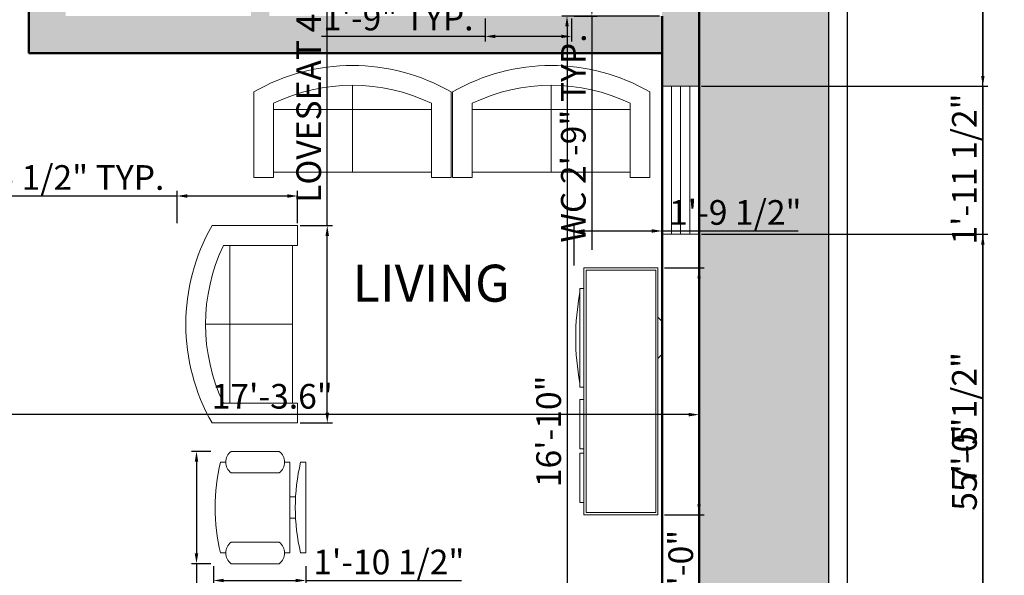
# Model space of a CAD drawing. Units: inches. Extents: x 2623 to 3157, y 1514 to 2273.
# Tile 5 of 6: x 2917 to 3157, y 1856 to 1991. Entities that reach past the tile are written whole.
import ezdxf

# ---------------------------------------------------------------- set-up
doc = ezdxf.new("R2010")
doc.units = ezdxf.units.IN
for name, color, linetype, lineweight in [('A-ANNO-DIMS', 2, 'Continuous', 18), ('A-AREA-IDEN', 7, 'Continuous', 25), ('A-FURN', 8, 'Continuous', 18), ('A-GLAZ', 4, 'Continuous', 20), ('A-WALL', 7, 'Continuous', 50), ('A-WALL-PATT', 252, 'Continuous', 13), ('C-PROP', 7, 'Continuous', 25), ('L-PLNT-PATT', 9, 'Continuous', 13)]:
    doc.layers.add(name, color=color, linetype=linetype, lineweight=lineweight)
doc.styles.get("Standard").update_dxf_attribs({"font": 'arial.ttf'})
doc.dimstyles.new('ISO-25', dxfattribs={"dimtxt": 6, "dimasz": 2.5, "dimexe": 1.25, "dimexo": 0.625, "dimtad": 1, "dimdec": 1, "dimlunit": 3, "dimtxsty": 'Standard', "dimcen": 2.5, "dimadec": 0, "dimazin": 0, "dimtfac": 1, "dimtdec": 1, "dimtmove": 0, "dimatfit": 3, "dimfxl": 1, "dimarcsym": 0})

# ---------------------------------------------------------------- blocks, each defined once
blk = doc.blocks.new('Sofa - Roundback Loveseat 5 ft.')
for p, q in [((0, -32.44198), (0, -5.99998)), ((-24, -33.99998), (-24, -11.46958)), ((24.00004, -33.99998), (24.00004, -11.46958)), ((-23.9998, -13.38178), (23.99986, -13.38178)), ((-24, -32.44198), (24.00004, -32.44198))]:
    blk.add_line(p, q)
for points in [[(-24, -33.99998), (-30, -33.99998), (-30, -7.99998)], [(30.00004, -7.99998), (30.00004, -33.99998), (24.00004, -33.99998)]]:
    blk.add_lwpolyline(points)
for centre, radius, start, end in [((0, -60.24998), 60.24998, 60.13715, 119.8628), ((0, -61.38438), 55.38444, 64.32083, 115.6792)]:
    blk.add_arc(centre, radius, start, end)
blk = doc.blocks.new('Chair - Desk')
for p, q in [((-8.5, 0), (-8.5, -1)), ((-8.5, 0), (8.5, 0)), ((8.5, 0), (8.5, -1)), ((-8.5, -3), (-8.5, -4)), ((-8.5, -3), (8.5, -3)), ((-2, -3), (-2, -1.9355)), ((2, -1.9576), (2, -3)), ((8.5, -3), (8.5, -4)), ((-10.5, -5), (-10.5, -14)), ((-6.5, -14), (-6.5, -5)), ((6.5, -5), (6.5, -14)), ((10.5, -14), (10.5, -5)), ((-8.5, -15), (-8.5, -16)), ((8.5, -15), (8.5, -16))]:
    blk.add_line(p, q)
for centre, radius, start, end in [((0, 34.625), 36.625, 256.5803, 283.4197), ((-8.5, -6.5), 2.5, 36.8699, 143.1301), ((8.5, -6.5), 2.5, 36.8699, 143.1301), ((-8.5, -12.5), 2.5, 216.8699, 323.1301), ((8.5, -12.5), 2.5, 216.8699, 323.1301), ((0, 19.625), 36.625, 256.5803, 283.4197)]:
    blk.add_arc(centre, radius, start, end)
blk = doc.blocks.new('Entertainment Center')
for p, q in [((-4, 0), (-5, -1)), ((4, 0), (-4, 0)), ((5, -1), (4, 0)), ((-17, -19), (-17, -1)), ((-17, -1), (43, -1)), ((-16.5, -18.5), (-16.5, -1.5)), ((-16.5, -1.5), (42.5, -1.5)), ((42.5, -1.5), (42.5, -18.5)), ((43, -1), (43, -19)), ((43, -19), (-17, -19)), ((42.5, -18.5), (-16.5, -18.5)), ((-12, -20), (-12, -19)), ((12, -19), (12, -20)), ((15, -20), (15, -19)), ((27, -19), (27, -20)), ((28, -20), (28, -19)), ((40, -19), (40, -20)), ((12, -20), (-12, -20)), ((27, -20), (15, -20)), ((40, -20), (28, -20))]:
    blk.add_line(p, q)
blk.add_arc((0, 40), 61, 259.6111, 280.3889)
blk = doc.blocks.new('Window - Wood Frame 36 in. Wide plan')
for p, q in [((0, 6), (0, 0)), ((36, 6), (36, 0)), ((0, 4.5), (36, 4.5)), ((0, 3), (36, 3)), ((0, 1.5), (36, 1.5))]:
    blk.add_line(p, q)
blk = doc.blocks.new('*D21')
at = {"layer": 'A-ANNO-DIMS', "color": 0, "lineweight": -2, "transparency": 16777216}
for p, q in [((3072.67, 1991.65), (3048.93, 1991.65)), ((3050.18, 1989.15), (3050.18, 1792.15)), ((3072.67, 1789.65), (3048.93, 1789.65))]:
    blk.add_line(p, q, dxfattribs=at)
at = {"layer": 'A-ANNO-DIMS', "color": 0, "transparency": 16777216}
for points in [[(3049.76, 1989.15), (3050.59, 1989.15), (3050.18, 1991.65)], [(3049.76, 1792.15), (3050.59, 1792.15), (3050.18, 1789.65)]]:
    blk.add_solid(points, dxfattribs=at)
at = {"layer": 'Defpoints', "color": 0, "transparency": 16777216}
for p in [(3073.3, 1991.65), (3050.18, 1789.65), (3073.3, 1789.65)]:
    blk.add_point(p, dxfattribs=at)
at = {"layer": 'A-ANNO-DIMS', "color": 0, "transparency": 16777216, "insert": (3046.49, 1890.65), "char_height": 6, "attachment_point": 5, "rotation": 90}
blk.add_mtext('16\'-10"', dxfattribs=at)
blk = doc.blocks.new('*D22')
at = {"layer": 'A-ANNO-DIMS', "color": 0, "lineweight": -2, "transparency": 16777216}
for p, q in [((2874.71, 1864.27), (2874.71, 1895.95)), ((3079.8, 1894.7), (2877.21, 1894.7)), ((3082.3, 1857.21), (3082.3, 1895.95))]:
    blk.add_line(p, q, dxfattribs=at)
at = {"layer": 'A-ANNO-DIMS', "color": 0, "transparency": 16777216}
for points in [[(2877.21, 1895.12), (2877.21, 1894.28), (2874.71, 1894.7)], [(3079.8, 1895.12), (3079.8, 1894.28), (3082.3, 1894.7)]]:
    blk.add_solid(points, dxfattribs=at)
at = {"layer": 'Defpoints', "color": 0, "transparency": 16777216}
for p in [(2874.71, 1894.7), (2874.71, 1863.65), (3082.3, 1856.59)]:
    blk.add_point(p, dxfattribs=at)
at = {"layer": 'A-ANNO-DIMS', "color": 0, "transparency": 16777216, "insert": (2978.5, 1898.39), "char_height": 6, "attachment_point": 5}
blk.add_mtext('17\'-3.6"', dxfattribs=at)
blk = doc.blocks.new('*D45')
at = {"layer": 'A-ANNO-DIMS', "color": 0, "lineweight": -2, "transparency": 16777216}
for p, q in [((2991.88, 1940.67), (2991.88, 2027.31)), ((2985.3, 1940.67), (2993.13, 1940.67)), ((2991.88, 1895.17), (2991.88, 1938.17)), ((2985.3, 1892.67), (2993.13, 1892.67))]:
    blk.add_line(p, q, dxfattribs=at)
at = {"layer": 'A-ANNO-DIMS', "color": 0, "transparency": 16777216}
for points in [[(2991.46, 1938.17), (2992.3, 1938.17), (2991.88, 1940.67)], [(2991.46, 1895.17), (2992.3, 1895.17), (2991.88, 1892.67)]]:
    blk.add_solid(points, dxfattribs=at)
at = {"layer": 'Defpoints', "color": 0, "transparency": 16777216}
for p in [(2984.68, 1940.67), (2991.88, 1940.67), (2984.68, 1892.67)]:
    blk.add_point(p, dxfattribs=at)
at = {"layer": 'A-ANNO-DIMS', "color": 0, "transparency": 16777216, "insert": (2988.15, 1985.24), "char_height": 6, "attachment_point": 5, "rotation": 90}
blk.add_mtext('LOVESEAT 4\'-0" TYP.', dxfattribs=at)
blk = doc.blocks.new('*D46')
at = {"layer": 'A-ANNO-DIMS', "color": 0, "lineweight": -2, "transparency": 16777216}
for p, q in [((2955.35, 1941.29), (2955.35, 1949.12)), ((2984.68, 1941.29), (2984.68, 1949.12)), ((2955.35, 1947.87), (2900.94, 1947.87)), ((2982.18, 1947.87), (2957.85, 1947.87))]:
    blk.add_line(p, q, dxfattribs=at)
at = {"layer": 'A-ANNO-DIMS', "color": 0, "transparency": 16777216}
for points in [[(2957.85, 1948.29), (2957.85, 1947.45), (2955.35, 1947.87)], [(2982.18, 1948.29), (2982.18, 1947.45), (2984.68, 1947.87)]]:
    blk.add_solid(points, dxfattribs=at)
at = {"layer": 'Defpoints', "color": 0, "transparency": 16777216}
for p in [(2955.35, 1947.87), (2955.35, 1940.67), (2984.68, 1940.67)]:
    blk.add_point(p, dxfattribs=at)
at = {"layer": 'A-ANNO-DIMS', "color": 0, "transparency": 16777216, "insert": (2926.89, 1951.6), "char_height": 6, "attachment_point": 5}
blk.add_mtext('2\'-5 1/2" TYP.', dxfattribs=at)
blk = doc.blocks.new('*D47')
at = {"layer": 'A-ANNO-DIMS', "color": 0, "lineweight": -2, "transparency": 16777216}
for p, q in [((3051.9, 2024.69), (3057.48, 2024.69)), ((3056.23, 2022.19), (3056.23, 1994.15)), ((3051.9, 1991.65), (3057.48, 1991.65)), ((3056.23, 1991.65), (3056.23, 1934.78))]:
    blk.add_line(p, q, dxfattribs=at)
at = {"layer": 'A-ANNO-DIMS', "color": 0, "transparency": 16777216}
for points in [[(3055.81, 2022.19), (3056.65, 2022.19), (3056.23, 2024.69)], [(3055.81, 1994.15), (3056.65, 1994.15), (3056.23, 1991.65)]]:
    blk.add_solid(points, dxfattribs=at)
at = {"layer": 'Defpoints', "color": 0, "transparency": 16777216}
for p in [(3051.27, 2024.69), (3051.27, 1991.65), (3056.23, 1991.65)]:
    blk.add_point(p, dxfattribs=at)
at = {"layer": 'A-ANNO-DIMS', "color": 0, "transparency": 16777216, "insert": (3052.5, 1961.97), "char_height": 6, "attachment_point": 5, "rotation": 90}
blk.add_mtext('WC 2\'-9" TYP.', dxfattribs=at)
blk = doc.blocks.new('*D48')
at = {"layer": 'A-ANNO-DIMS', "color": 0, "lineweight": -2, "transparency": 16777216}
for p, q in [((3030.27, 1991.02), (3030.27, 1985.44)), ((3051.27, 1991.02), (3051.27, 1985.44)), ((3030.27, 1986.69), (2990.51, 1986.69)), ((3048.77, 1986.69), (3032.77, 1986.69))]:
    blk.add_line(p, q, dxfattribs=at)
at = {"layer": 'A-ANNO-DIMS', "color": 0, "transparency": 16777216}
for points in [[(3032.77, 1987.11), (3032.77, 1986.27), (3030.27, 1986.69)], [(3048.77, 1987.11), (3048.77, 1986.27), (3051.27, 1986.69)]]:
    blk.add_solid(points, dxfattribs=at)
at = {"layer": 'Defpoints', "color": 0, "transparency": 16777216}
for p in [(3030.27, 1991.65), (3051.27, 1991.65), (3030.27, 1986.69)]:
    blk.add_point(p, dxfattribs=at)
at = {"layer": 'A-ANNO-DIMS', "color": 0, "transparency": 16777216, "insert": (3009.14, 1990.38), "char_height": 6, "attachment_point": 5}
blk.add_mtext('1\'-9" TYP.', dxfattribs=at)
blk = doc.blocks.new('*D51')
at = {"layer": 'A-ANNO-DIMS', "color": 0, "lineweight": -2, "transparency": 16777216}
for p, q in [((2963.55, 1885.76), (2958.83, 1885.76)), ((2960.08, 1883.26), (2960.08, 1860.96)), ((2963.55, 1858.46), (2958.83, 1858.46)), ((2960.08, 1858.46), (2960.08, 1771.51))]:
    blk.add_line(p, q, dxfattribs=at)
at = {"layer": 'A-ANNO-DIMS', "color": 0, "transparency": 16777216}
for points in [[(2959.66, 1883.26), (2960.5, 1883.26), (2960.08, 1885.76)], [(2959.66, 1860.96), (2960.5, 1860.96), (2960.08, 1858.46)]]:
    blk.add_solid(points, dxfattribs=at)
at = {"layer": 'Defpoints', "color": 0, "transparency": 16777216}
for p in [(2964.18, 1885.76), (2960.08, 1858.46), (2964.18, 1858.46)]:
    blk.add_point(p, dxfattribs=at)
at = {"layer": 'A-ANNO-DIMS', "color": 0, "transparency": 16777216, "insert": (2956.35, 1813.73), "char_height": 6, "attachment_point": 5, "rotation": 90}
blk.add_mtext('DESK CHAIR 2\'-3 1/2"', dxfattribs=at)
blk = doc.blocks.new('*D52')
at = {"layer": 'A-ANNO-DIMS', "color": 0, "lineweight": -2, "transparency": 16777216}
for p, q in [((2964.18, 1857.83), (2964.18, 1853.11)), ((2986.71, 1857.83), (2986.71, 1853.11)), ((2966.68, 1854.36), (2984.21, 1854.36)), ((2986.71, 1854.36), (3024.49, 1854.36))]:
    blk.add_line(p, q, dxfattribs=at)
at = {"layer": 'A-ANNO-DIMS', "color": 0, "transparency": 16777216}
for points in [[(2966.68, 1854.78), (2966.68, 1853.95), (2964.18, 1854.36)], [(2984.21, 1854.78), (2984.21, 1853.95), (2986.71, 1854.36)]]:
    blk.add_solid(points, dxfattribs=at)
at = {"layer": 'Defpoints', "color": 0, "transparency": 16777216}
for p in [(2964.18, 1858.46), (2986.71, 1858.46), (2986.71, 1854.36)]:
    blk.add_point(p, dxfattribs=at)
at = {"layer": 'A-ANNO-DIMS', "color": 0, "transparency": 16777216, "insert": (3006.85, 1858.09), "char_height": 6, "attachment_point": 5}
blk.add_mtext('1\'-10 1/2"', dxfattribs=at)
blk = doc.blocks.new('*D53')
at = {"layer": 'A-ANNO-DIMS', "color": 0, "lineweight": -2, "transparency": 16777216}
for p, q in [((3073.92, 1930.37), (3083.55, 1930.37)), ((3082.3, 1927.87), (3082.3, 1872.87)), ((3073.92, 1870.37), (3083.55, 1870.37)), ((3082.3, 1870.37), (3082.3, 1800.19))]:
    blk.add_line(p, q, dxfattribs=at)
at = {"layer": 'A-ANNO-DIMS', "color": 0, "transparency": 16777216}
for points in [[(3081.88, 1927.87), (3082.71, 1927.87), (3082.3, 1930.37)], [(3081.88, 1872.87), (3082.71, 1872.87), (3082.3, 1870.37)]]:
    blk.add_solid(points, dxfattribs=at)
at = {"layer": 'Defpoints', "color": 0, "transparency": 16777216}
for p in [(3073.3, 1930.37), (3073.3, 1870.37), (3082.3, 1870.37)]:
    blk.add_point(p, dxfattribs=at)
at = {"layer": 'A-ANNO-DIMS', "color": 0, "transparency": 16777216, "insert": (3078.61, 1834.03), "char_height": 6, "attachment_point": 5, "rotation": 90}
blk.add_mtext('MEDIA UNIT 5\'-0"', dxfattribs=at)
blk = doc.blocks.new('*D54')
at = {"layer": 'A-ANNO-DIMS', "color": 0, "lineweight": -2, "transparency": 16777216}
for p, q in [((3051.96, 1931), (3051.96, 1940.62)), ((3054.46, 1939.37), (3070.8, 1939.37)), ((3073.3, 1931), (3073.3, 1940.62)), ((3073.3, 1939.37), (3106.41, 1939.37))]:
    blk.add_line(p, q, dxfattribs=at)
at = {"layer": 'A-ANNO-DIMS', "color": 0, "transparency": 16777216}
for points in [[(3054.46, 1939.79), (3054.46, 1938.95), (3051.96, 1939.37)], [(3070.8, 1939.79), (3070.8, 1938.95), (3073.3, 1939.37)]]:
    blk.add_solid(points, dxfattribs=at)
at = {"layer": 'Defpoints', "color": 0, "transparency": 16777216}
for p in [(3073.3, 1939.37), (3051.96, 1930.37), (3073.3, 1930.37)]:
    blk.add_point(p, dxfattribs=at)
at = {"layer": 'A-ANNO-DIMS', "color": 0, "transparency": 16777216, "insert": (3091.1, 1943.1), "char_height": 6, "attachment_point": 5}
blk.add_mtext('1\'-9 1/2"', dxfattribs=at)
blk = doc.blocks.new('*D60')
at = {"layer": 'A-ANNO-DIMS', "color": 0, "lineweight": -2, "transparency": 16777216}
for p, q in [((3118.92, 2212.65), (3152.55, 2212.65)), ((3151.3, 1555.15), (3151.3, 2210.15)), ((3118.92, 1552.65), (3152.55, 1552.65))]:
    blk.add_line(p, q, dxfattribs=at)
at = {"layer": 'A-ANNO-DIMS', "color": 0, "transparency": 16777216}
for points in [[(3150.88, 2210.15), (3151.71, 2210.15), (3151.3, 2212.65)], [(3150.88, 1555.15), (3151.71, 1555.15), (3151.3, 1552.65)]]:
    blk.add_solid(points, dxfattribs=at)
at = {"layer": 'Defpoints', "color": 0, "transparency": 16777216}
for p in [(3118.3, 2212.65), (3151.3, 2212.65), (3118.3, 1552.65)]:
    blk.add_point(p, dxfattribs=at)
at = {"layer": 'A-ANNO-DIMS', "color": 0, "transparency": 16777216, "insert": (3147.61, 1882.65), "char_height": 6, "attachment_point": 5, "rotation": 90}
blk.add_mtext('55\'-0"', dxfattribs=at)
blk = doc.blocks.new('*D94')
at = {"layer": 'A-ANNO-DIMS', "color": 0, "lineweight": -2, "transparency": 16777216}
for p, q in [((3082.92, 1998.16), (3152.55, 1998.16)), ((3151.3, 1995.66), (3151.3, 1977.07)), ((3082.92, 1974.57), (3152.55, 1974.57)), ((3151.3, 1974.57), (3151.3, 1936.8))]:
    blk.add_line(p, q, dxfattribs=at)
at = {"layer": 'A-ANNO-DIMS', "color": 0, "transparency": 16777216}
for points in [[(3150.88, 1995.66), (3151.71, 1995.66), (3151.3, 1998.16)], [(3150.88, 1977.07), (3151.71, 1977.07), (3151.3, 1974.57)]]:
    blk.add_solid(points, dxfattribs=at)
at = {"layer": 'Defpoints', "color": 0, "transparency": 16777216}
for p in [(3082.3, 1998.16), (3082.3, 1974.57), (3151.3, 1974.57)]:
    blk.add_point(p, dxfattribs=at)
at = {"layer": 'A-ANNO-DIMS', "color": 0, "transparency": 16777216, "insert": (3147.57, 1954.44), "char_height": 6, "attachment_point": 5, "rotation": 90}
blk.add_mtext('1\'-11 1/2"', dxfattribs=at)
blk = doc.blocks.new('*D95')
at = {"layer": 'A-ANNO-DIMS', "color": 0, "lineweight": -2, "transparency": 16777216}
for p, q in [((3082.92, 1938.57), (3152.55, 1938.57)), ((3151.3, 1936.07), (3151.3, 1851.59)), ((3082.92, 1849.09), (3152.55, 1849.09))]:
    blk.add_line(p, q, dxfattribs=at)
at = {"layer": 'A-ANNO-DIMS', "color": 0, "transparency": 16777216}
for points in [[(3150.88, 1936.07), (3151.71, 1936.07), (3151.3, 1938.57)], [(3150.88, 1851.59), (3151.71, 1851.59), (3151.3, 1849.09)]]:
    blk.add_solid(points, dxfattribs=at)
at = {"layer": 'Defpoints', "color": 0, "transparency": 16777216}
for p in [(3082.3, 1938.57), (3082.3, 1849.09), (3151.3, 1849.09)]:
    blk.add_point(p, dxfattribs=at)
at = {"layer": 'A-ANNO-DIMS', "color": 0, "transparency": 16777216, "insert": (3147.57, 1893.83), "char_height": 6, "attachment_point": 5, "rotation": 90}
blk.add_mtext('7\'-5 1/2"', dxfattribs=at)

msp = doc.modelspace()

# ---------------------------------------------------------------- hatches: boundary and pattern name
at = {"layer": 'A-WALL-PATT'}
h = msp.add_hatch(color=256, dxfattribs=at)
h.dxf.hatch_style = 1
h.paths.add_polyline_path([(2704.3, 1854.65), (2893.38, 1854.65), (2893.38, 1850.02), (2902.38, 1850.02), (2902.38, 1863.65), (2704.3, 1863.65), (2704.3, 1949.25), (2695.3, 1949.25), (2695.3, 1845.57), (2704.3, 1845.57)])
h.paths.add_polyline_path([(2704.3, 1809.57), (2695.3, 1809.57), (2695.3, 1750.74), (2704.3, 1750.74)])
h.paths.add_polyline_path([(2764.7, 1621.65), (2704.3, 1621.65), (2704.3, 1660.74), (2695.3, 1660.74), (2695.3, 1612.65), (2764.7, 1612.65)])
h.paths.add_polyline_path([(2704.3, 2128.1), (2695.3, 2128.1), (2695.3, 2039.25), (2704.3, 2039.25)])
h.paths.add_polyline_path([(2714, 2185.65), (2695.3, 2185.65), (2695.3, 2164.1), (2704.3, 2164.1), (2704.3, 2176.65), (2714, 2176.65)])
h.paths.add_polyline_path([(2797.66, 2185.65), (2768, 2185.65), (2768, 2176.65), (2797.66, 2176.65)])
h.paths.add_polyline_path([(2777.8, 2176.65), (2773.3, 2176.65), (2773.3, 2142.65), (2777.8, 2142.65)])
h.paths.add_polyline_path([(2963.13, 2185.65), (2887.66, 2185.65), (2887.66, 2176.65), (2963.13, 2176.65)])
h.paths.add_polyline_path([(2928.3, 2176.65), (2919.3, 2176.65), (2919.3, 2047.65), (2850.8, 2047.65), (2850.8, 2038.65), (2919.3, 2038.65), (2919.3, 2031.57), (2928.3, 2031.57), (2928.3, 2038.65)])
h.paths.add_polyline_path([(3082.3, 2185.65), (3053.13, 2185.65), (3053.13, 2176.65), (3073.3, 2176.65), (3073.3, 2169.26), (3082.3, 2169.26)])
h.paths.add_polyline_path([(3082.3, 2133.26), (3073.3, 2133.26), (3073.3, 2047.65), (2977.8, 2047.65), (2977.8, 2074.51), (2973.3, 2074.51), (2973.3, 2047.65), (2973.3, 2038.65), (2973.3, 2021.33), (2977.8, 2021.33), (2977.8, 2038.65), (3005.74, 2038.65, -0.027912), (3007.41, 2038.69, -0.0118), (3008.11, 2038.65), (3073.3, 2038.65), (3073.3, 2034.16), (3082.3, 2034.16)])
h.paths.add_polyline_path([(3082.3, 1998.16), (3073.3, 1998.16), (3073.3, 1991.65), (2977.8, 1991.65), (2977.8, 1997.33), (2973.3, 1997.33), (2973.3, 1991.65), (2928.3, 1991.65), (2928.3, 1995.57), (2919.3, 1995.57), (2919.3, 1982.65), (3073.3, 1982.65), (3073.3, 1974.57), (3082.3, 1974.57)])
at = {"layer": 'L-PLNT-PATT'}
h = msp.add_hatch(color=256, dxfattribs=at)
h.dxf.hatch_style = 1
h.set_gradient(color1=(19, 155, 72), color2=(63, 255, 0), name='CURVED')
h.paths.add_polyline_path([(2902.38, 1612.65), (2695.3, 1612.65), (2695.3, 2185.65), (3082.3, 2185.65), (3082.3, 1780.65), (3113.8, 1780.65), (3113.8, 2208.15), (2672.8, 2208.15), (2672.8, 1557.15), (2902.38, 1557.15)])
h = msp.add_hatch(color=256, dxfattribs=at)
h.dxf.hatch_style = 1
h.set_gradient(color1=(19, 155, 72), color2=(63, 255, 0), name='CYLINDER')
h.paths.add_polyline_path([(3024.32, 1726.09), (2994.86, 1726.09), (2994.86, 1587.38), (3024.32, 1587.38)], flags=17)
h.paths.add_polyline_path([(2902.38, 1612.65), (2695.3, 1612.65), (2695.3, 2185.65), (3082.3, 2185.65), (3082.3, 1780.65), (3113.8, 1780.65), (3113.8, 2208.15), (2672.8, 2208.15), (2672.8, 1557.15), (2902.38, 1557.15)])

# ---------------------------------------------------------------- linework, layer by layer
at = {"layer": 'A-GLAZ'}
for p, q in [((3073.3, 1974.57), (3082.3, 1974.57)), ((3073.3, 1938.57), (3082.3, 1938.57))]:
    msp.add_line(p, q, dxfattribs=at)
at = {"layer": 'A-WALL'}
for p, q in [((3082.3, 2185.65), (3082.3, 1780.65)), ((2919.3, 1982.65), (2919.3, 1995.57)), ((3073.3, 1991.65), (3073.3, 1789.65)), ((2919.3, 1982.65), (3073.3, 1982.65)), ((3073.3, 1982.65), (3073.3, 1789.65))]:
    msp.add_line(p, q, dxfattribs=at)
at = {"layer": 'C-PROP'}
for p, q in [((3118.3, 2212.65), (3118.3, 1552.65)), ((3113.8, 2208.15), (3113.8, 1557.15))]:
    msp.add_line(p, q, dxfattribs=at)

# ---------------------------------------------------------------- block references
at = {"layer": 'A-FURN', "xscale": 0.8, "yscale": 0.8}
for p in [(2998.01, 1979.6), (3046.33, 1979.6)]:
    msp.add_blockref('Sofa - Roundback Loveseat 5 ft.', p, dxfattribs=at)
at = {"layer": 'A-FURN'}
for name, p, xscale, yscale, rotation in [('Sofa - Roundback Loveseat 5 ft.', (2957.48, 1916.67), 0.8, 0.8, 90), ('Chair - Desk', (2986.71, 1872.11), 1.3, 1.3, 270)]:
    msp.add_blockref(name, p, dxfattribs=dict(at, xscale=xscale, yscale=yscale, rotation=rotation))
at = {"layer": 'A-FURN', "rotation": 270}
msp.add_blockref('Entertainment Center', (3073.3, 1913.37), dxfattribs=at)
at = {"layer": 'A-GLAZ', "yscale": 1.5, "rotation": 90}
msp.add_blockref('Window - Wood Frame 36 in. Wide plan', (3082.3, 1938.57), dxfattribs=at)

# ---------------------------------------------------------------- texts
at = {"layer": 'A-AREA-IDEN', "insert": (2998.02, 1931.17), "char_height": 9, "attachment_point": 1}
msp.add_mtext('LIVING', dxfattribs=at)

# ---------------------------------------------------------------- dimensions: what is measured, and where the dimension line sits
at = {"layer": 'A-ANNO-DIMS'}
for base, p1, p2, override, picture, middle in [((3151.3, 2212.65), (3118.3, 1552.65), (3118.3, 2212.65), {"dimdec": 1, "dimlfac": 1, "dimrnd": 0, "dimzin": 1, "dimdsep": 46, "dimlunit": 4, "dimfrac": 2}, '*D60', (3147.61, 1882.65)), ((3151.3, 1974.57), (3082.3, 1998.16), (3082.3, 1974.57), {"dimdec": 1, "dimlfac": 1, "dimrnd": 0, "dimzin": 1, "dimdsep": 46, "dimlunit": 4, "dimfrac": 2}, '*D94', (3147.57, 1954.44)), ((3050.18, 1789.65), (3073.3, 1991.65), (3073.3, 1789.65), {"dimclrd": 0, "dimclre": 0, "dimclrt": 0}, '*D21', (3046.49, 1890.65)), ((3151.3, 1849.09), (3082.3, 1938.57), (3082.3, 1849.09), {"dimdec": 1, "dimlfac": 1, "dimrnd": 0, "dimzin": 1, "dimdsep": 46, "dimlunit": 4, "dimfrac": 2}, '*D95', (3147.57, 1893.83))]:
    dim = msp.add_linear_dim(base=base, p1=p1, p2=p2, angle=90, dimstyle='ISO-25', override=override, dxfattribs=at)
    dim.commit()
    dim.dimension.update_dxf_attribs({"geometry": picture, "text_midpoint": middle})
for base, p1, p2, angle, text, picture, middle in [((2991.88, 1940.67), (2984.68, 1892.67), (2984.68, 1940.67), 90, 'LOVESEAT <> TYP.', '*D45', (2988.15, 1985.24)), ((3056.23, 1991.65), (3051.27, 2024.69), (3051.27, 1991.65), 270, 'WC <> TYP.', '*D47', (3052.5, 1961.97)), ((3030.27, 1986.69), (3051.27, 1991.65), (3030.27, 1991.65), 180, '<> TYP.', '*D48', (3009.14, 1990.38)), ((2955.35, 1947.87), (2984.68, 1940.67), (2955.35, 1940.67), 180, '<> TYP.', '*D46', (2926.89, 1951.6)), ((3082.3, 1870.37), (3073.3, 1930.37), (3073.3, 1870.37), 270, 'MEDIA UNIT <>', '*D53', (3078.61, 1834.03)), ((2960.08, 1858.46), (2964.18, 1885.76), (2964.18, 1858.46), 270, 'DESK CHAIR <>', '*D51', (2956.35, 1813.73))]:
    dim = msp.add_linear_dim(base=base, p1=p1, p2=p2, angle=angle, text=text, dimstyle='ISO-25', override={"dimdec": 1, "dimlfac": 1, "dimrnd": 0, "dimzin": 1, "dimdsep": 46, "dimlunit": 4, "dimfrac": 2}, dxfattribs=at)
    dim.commit()
    dim.dimension.update_dxf_attribs({"geometry": picture, "text_midpoint": middle})
for base, p1, p2, override, picture, middle in [((3073.3, 1939.37), (3051.96, 1930.37), (3073.3, 1930.37), {"dimdec": 1, "dimlfac": 1, "dimrnd": 0, "dimzin": 1, "dimdsep": 46, "dimlunit": 4, "dimfrac": 2}, '*D54', (3091.1, 1943.1)), ((2874.71, 1894.7), (3082.3, 1856.59), (2874.71, 1863.65), {"dimclrd": 0, "dimclre": 0, "dimclrt": 0}, '*D22', (2978.5, 1898.39)), ((2986.71, 1854.36), (2964.18, 1858.46), (2986.71, 1858.46), {"dimdec": 1, "dimlfac": 1, "dimrnd": 0, "dimzin": 1, "dimdsep": 46, "dimlunit": 4, "dimfrac": 2}, '*D52', (3006.85, 1858.09))]:
    dim = msp.add_linear_dim(base=base, p1=p1, p2=p2, dimstyle='ISO-25', override=override, dxfattribs=at)
    dim.commit()
    dim.dimension.update_dxf_attribs({"geometry": picture, "text_midpoint": middle})

doc.saveas('drawing.dxf')
